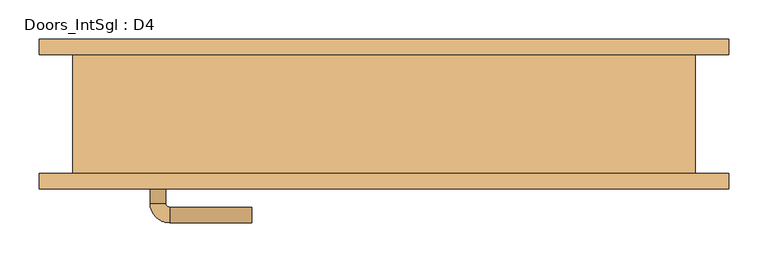
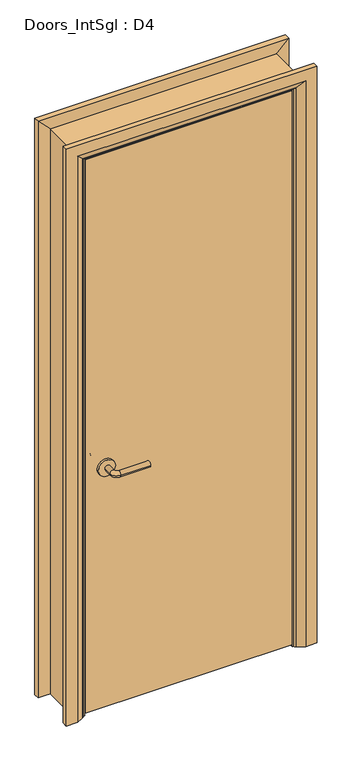
"""IFC4 building model written with IfcOpenShell, lengths in millimetres: door geometry, Doors_IntSgl : D4."""

from ifc_helpers import new_model, si_unit, point, frame, frame_2d, origin, place, context, project, spatial, polyline, circle_curve, ellipse_curve, trimmed, segment, composite_curve, outline, extrude, faceted_brep, source, transform, mapped, element, save
from ifc_brep_helpers import plane_surface, cylinder_surface, revolved_surface, advanced_brep


def doors_intsgl_d4_c85c0d06(model_context):
    return source(origin(), model_context, "Body", "SolidModel", [
        advanced_brep(
        [(-299.4508, -30.2, 900.0), (-279.4508, -30.2, 900.0), (-299.4508, -0.2, 900.0), (-279.4508, -0.2, 900.0), (-274.4508, 4.8, 900.0), (-274.4508, 24.8, 900.0), (-169.4508, 24.8, 900.0), (-169.4508, 4.8, 900.0)],
        [
            (0, 1, circle_curve(frame((-289.4508, -30.2, 900.0), z_axis=(0.0, -1.0, 0.0), x_axis=(1.0, 0.0, 0.0)), 10.0)),
            (1, 0, circle_curve(frame((-289.4508, -30.2, 900.0), z_axis=(0.0, -1.0, 0.0), x_axis=(1.0, 0.0, 0.0)), 10.0)),
            (0, 2),
            (2, 3, circle_curve(frame((-289.4508, -0.2, 900.0), z_axis=(0.0, -1.0, 0.0), x_axis=(1.0, 0.0, 0.0)), 10.0)),
            (3, 1),
            (3, 2, circle_curve(frame((-289.4508, -0.2, 900.0), z_axis=(0.0, -1.0, 0.0), x_axis=(1.0, 0.0, 0.0)), 10.0)),
            (4, 3, circle_curve(frame((-274.4508, -0.2, 900.0), z_axis=(0.0, 0.0, 1.0), x_axis=(-1.0, 0.0, 0.0)), 5.0)),
            (2, 5, circle_curve(frame((-274.4508, -0.2, 900.0), z_axis=(0.0, 0.0, -1.0), x_axis=(-1.0, 0.0, 0.0)), 25.0)),
            (5, 4, circle_curve(frame((-274.4508, 14.8, 900.0), z_axis=(-1.0, 0.0, 0.0), x_axis=(0.0, -1.0, 0.0)), 10.0)),
            (4, 5, circle_curve(frame((-274.4508, 14.8, 900.0), z_axis=(-1.0, 0.0, 0.0), x_axis=(0.0, -1.0, 0.0)), 10.0)),
            (6, 7, circle_curve(frame((-169.4508, 14.8, 900.0), z_axis=(1.0, 0.0, 0.0), x_axis=(0.0, -1.0, 0.0)), 10.0)),
            (7, 6, circle_curve(frame((-169.4508, 14.8, 900.0), z_axis=(1.0, 0.0, 0.0), x_axis=(0.0, -1.0, 0.0)), 10.0)),
            (5, 6),
            (7, 4),
        ],
        [
            plane_surface(frame((-289.4508, -30.2, 900.0), z_axis=(0.0, -1.0, 0.0), x_axis=(0.0, 0.0, 1.0))),
            cylinder_surface(frame((-289.4508, -30.2, 900.0), z_axis=(0.0, -1.0, 0.0), x_axis=(1.0, 0.0, 0.0)), 10.0),
            revolved_surface(trimmed(ellipse_curve(frame((-289.4508, -0.2, 900.0), z_axis=(0.0, -1.0, 0.0), x_axis=(1.0, 0.0, 0.0)), 10.0, 10.0), [point((-299.4508, -0.2, 900.0))], [point((-279.4508, -0.2, 900.0))], True, "CARTESIAN"), (-274.4508, -0.2, 900.0), (0.0, 0.0, -1.0)),
            revolved_surface(trimmed(ellipse_curve(frame((-289.4508, -0.2, 900.0), z_axis=(0.0, -1.0, 0.0), x_axis=(1.0, 0.0, 0.0)), 10.0, 10.0), [point((-279.4508, -0.2, 900.0))], [point((-299.4508, -0.2, 900.0))], True, "CARTESIAN"), (-274.4508, -0.2, 900.0), (0.0, 0.0, -1.0)),
            plane_surface(frame((-169.4508, 14.8, 900.0), z_axis=(1.0, 0.0, 0.0), x_axis=(0.0, 0.0, 1.0))),
            cylinder_surface(frame((-274.4508, 14.8, 900.0), z_axis=(-1.0, 0.0, 0.0), x_axis=(0.0, -1.0, 0.0)), 10.0),
        ],
        [
            (0, [[1, 2]]),
            (1, [[-1, 3, 4, 5]]),
            (1, [[-2, -5, 6, -3]]),
            (2, [[7, -4, 8, 9]]),
            (3, [[-8, -6, -7, 10]]),
            (4, [[11, 12]]),
            (5, [[-9, 13, -12, 14]]),
            (5, [[-10, -14, -11, -13]]),
        ],
    ),
        extrude(outline(composite_curve([segment(trimmed(circle_curve(frame_2d((900.0, -291.9508)), 30.0), [point((900.0, -321.9508))], [point((900.0, -261.9508))], False, "CARTESIAN"), True, "CONTINUOUS"), segment(trimmed(circle_curve(frame_2d((900.0, -291.9508)), 30.0), [point((900.0, -261.9508))], [point((900.0, -321.9508))], False, "CARTESIAN"), True, "CONTINUOUS")], self_intersect=False)), frame((0.0, -38.2, 0.0), z_axis=(0.0, 1.0, 0.0), x_axis=(0.0, 0.0, 1.0)), (0.0, 0.0, 1.0), 8.0),
        advanced_brep(
        [(-299.4508, -84.2, 900.0), (-279.4508, -84.2, 900.0), (-279.4508, -114.2, 900.0), (-299.4508, -114.2, 900.0), (-274.4508, -119.2, 900.0), (-274.4508, -139.2, 900.0), (-169.4508, -139.2, 900.0), (-169.4508, -119.2, 900.0)],
        [
            (0, 1, circle_curve(frame((-289.4508, -84.2, 900.0), z_axis=(0.0, 1.0, 0.0), x_axis=(1.0, 0.0, 0.0)), 10.0)),
            (1, 0, circle_curve(frame((-289.4508, -84.2, 900.0), z_axis=(0.0, 1.0, 0.0), x_axis=(1.0, 0.0, 0.0)), 10.0)),
            (1, 2),
            (2, 3, circle_curve(frame((-289.4508, -114.2, 900.0), z_axis=(0.0, 1.0, 0.0), x_axis=(1.0, 0.0, 0.0)), 10.0)),
            (3, 0),
            (3, 2, circle_curve(frame((-289.4508, -114.2, 900.0), z_axis=(0.0, 1.0, 0.0), x_axis=(1.0, 0.0, 0.0)), 10.0)),
            (4, 5, circle_curve(frame((-274.4508, -129.2, 900.0), z_axis=(-1.0, 0.0, 0.0), x_axis=(0.0, 1.0, 0.0)), 10.0)),
            (5, 3, circle_curve(frame((-274.4508, -114.2, 900.0), z_axis=(0.0, 0.0, -1.0), x_axis=(-1.0, 0.0, 0.0)), 25.0)),
            (2, 4, circle_curve(frame((-274.4508, -114.2, 900.0), z_axis=(0.0, 0.0, 1.0), x_axis=(-1.0, 0.0, 0.0)), 5.0)),
            (5, 4, circle_curve(frame((-274.4508, -129.2, 900.0), z_axis=(-1.0, 0.0, 0.0), x_axis=(0.0, 1.0, 0.0)), 10.0)),
            (6, 7, circle_curve(frame((-169.4508, -129.2, 900.0), z_axis=(1.0, 0.0, 0.0), x_axis=(0.0, 1.0, 0.0)), 10.0)),
            (7, 6, circle_curve(frame((-169.4508, -129.2, 900.0), z_axis=(1.0, 0.0, 0.0), x_axis=(0.0, 1.0, 0.0)), 10.0)),
            (4, 7),
            (6, 5),
        ],
        [
            plane_surface(frame((-289.4508, -84.2, 900.0), z_axis=(0.0, 1.0, 0.0), x_axis=(0.0, 0.0, 1.0))),
            cylinder_surface(frame((-289.4508, -84.2, 900.0), z_axis=(0.0, 1.0, 0.0), x_axis=(1.0, 0.0, 0.0)), 10.0),
            revolved_surface(trimmed(ellipse_curve(frame((-289.4508, -114.2, 900.0), z_axis=(0.0, -1.0, 0.0), x_axis=(1.0, 0.0, 0.0)), 10.0, 10.0), [point((-299.4508, -114.2, 900.0))], [point((-279.4508, -114.2, 900.0))], True, "CARTESIAN"), (-274.4508, -114.2, 900.0), (0.0, 0.0, -1.0)),
            revolved_surface(trimmed(ellipse_curve(frame((-289.4508, -114.2, 900.0), z_axis=(0.0, -1.0, 0.0), x_axis=(1.0, 0.0, 0.0)), 10.0, 10.0), [point((-279.4508, -114.2, 900.0))], [point((-299.4508, -114.2, 900.0))], True, "CARTESIAN"), (-274.4508, -114.2, 900.0), (0.0, 0.0, -1.0)),
            plane_surface(frame((-169.4508, -129.2, 900.0), z_axis=(1.0, 0.0, 0.0), x_axis=(0.0, 0.0, 1.0))),
            cylinder_surface(frame((-274.4508, -129.2, 900.0), z_axis=(-1.0, 0.0, 0.0), x_axis=(0.0, 1.0, 0.0)), 10.0),
        ],
        [
            (0, [[1, 2]]),
            (1, [[3, 4, 5, -2]]),
            (1, [[-5, 6, -3, -1]]),
            (2, [[7, 8, -4, 9]]),
            (3, [[10, -9, -6, -8]]),
            (4, [[11, 12]]),
            (5, [[13, -11, 14, -7]]),
            (5, [[-14, -12, -13, -10]]),
        ],
    ),
        extrude(outline(composite_curve([segment(trimmed(circle_curve(frame_2d((900.0, -291.9508)), 30.0), [point((900.0, -321.9508))], [point((900.0, -261.9508))], False, "CARTESIAN"), True, "CONTINUOUS"), segment(trimmed(circle_curve(frame_2d((900.0, -291.9508)), 30.0), [point((900.0, -261.9508))], [point((900.0, -321.9508))], False, "CARTESIAN"), True, "CONTINUOUS")], self_intersect=False)), frame((0.0, -84.2, 0.0), z_axis=(0.0, 1.0, 0.0), x_axis=(0.0, 0.0, 1.0)), (0.0, 0.0, 1.0), 8.0),
        extrude(outline(polyline([(364.4508, -38.2), (364.4508, -76.2), (-364.4508, -76.2), (-364.4508, -38.2), (364.4508, -38.2)])), frame((0.0, 0.0, 8.0), z_axis=(0.0, 0.0, 1.0), x_axis=(1.0, 0.0, 0.0)), (0.0, 0.0, 1.0), 2060.0),
        advanced_brep(
        [(441.4508, -96.2, 0.0), (401.4508, -96.2, 0.0), (375.4508, -82.2, 0.0), (371.4508, -76.2, 0.0), (441.4508, -76.2, 0.0), (441.4508, -76.2, 2145.0), (441.4508, -96.2, 2145.0), (371.4508, -76.2, 2075.0), (-371.4508, -76.2, 2075.0), (-371.4508, -76.2, 0.0), (-441.4508, -76.2, 0.0), (-441.4508, -76.2, 2145.0), (375.4508, -82.2, 2079.0), (401.4508, -96.2, 2105.0), (-441.4508, -96.2, 2145.0), (-441.4508, -96.2, 0.0), (-401.4508, -96.2, 0.0), (-401.4508, -96.2, 2105.0), (-375.4508, -82.2, 0.0), (-375.4508, -82.2, 2079.0)],
        [
            (0, 1),
            (1, 2),
            (2, 3, circle_curve(frame((379.4508, -75.2, 0.0), z_axis=(0.0, 0.0, -1.0), x_axis=(1.0, 0.0, 0.0)), 8.0622577)),
            (3, 4),
            (4, 0),
            (4, 5),
            (5, 6),
            (6, 0),
            (3, 7),
            (7, 8),
            (8, 9),
            (9, 10),
            (10, 11),
            (11, 5),
            (2, 12),
            (12, 7, ellipse_curve(frame((379.4508, -75.2, 2083.0), z_axis=(0.7071067811865475, 0.0, -0.7071067811865475), x_axis=(-0.7071067811865474, 0.0, -0.7071067811865476)), 11.4017543, 8.0622577)),
            (1, 13),
            (13, 12),
            (6, 14),
            (14, 15),
            (15, 16),
            (16, 17),
            (17, 13),
            (10, 15),
            (14, 11),
            (9, 18, circle_curve(frame((-379.4508, -75.2, 0.0), z_axis=(0.0, 0.0, -1.0), x_axis=(-1.0, 0.0, 0.0)), 8.0622577)),
            (18, 16),
            (19, 18),
            (8, 19, ellipse_curve(frame((-379.4508, -75.2, 2083.0), z_axis=(-0.7071067811865475, 0.0, -0.7071067811865475), x_axis=(-0.7071067811865474, 0.0, 0.7071067811865476)), 11.4017543, 8.0622577)),
            (19, 17),
            (12, 19),
        ],
        [
            plane_surface(frame((371.4508, -76.2, 0.0), z_axis=(0.0, 0.0, -1.0), x_axis=(0.0, 1.0, 0.0))),
            plane_surface(frame((441.4508, -96.2, 0.0), z_axis=(1.0, 0.0, 0.0), x_axis=(0.0, 0.0, 1.0))),
            plane_surface(frame((441.4508, -76.2, 0.0), z_axis=(0.0, 1.0, 0.0), x_axis=(0.0, 0.0, 1.0))),
            cylinder_surface(frame((379.4508, -75.2, 0.0), z_axis=(0.0, 0.0, -1.0), x_axis=(1.0, 0.0, 0.0)), 8.0622577),
            plane_surface(frame((375.4508, -82.2, 0.0), z_axis=(-0.4740998230350126, -0.880471099922178, 0.0), x_axis=(0.0, 0.0, 1.0))),
            plane_surface(frame((401.4508, -96.2, 0.0), z_axis=(0.0, -1.0, 0.0), x_axis=(0.0, 0.0, 1.0))),
            plane_surface(frame((-441.4508, -96.2, 2145.0), z_axis=(-1.0, 0.0, 0.0), x_axis=(0.0, 0.0, -1.0))),
            plane_surface(frame((-371.4508, -76.2, 0.0), z_axis=(0.0, 0.0, -1.0), x_axis=(0.0, 1.0, 0.0))),
            cylinder_surface(frame((-379.4508, -75.2, 2075.0), z_axis=(0.0, 0.0, 1.0), x_axis=(-1.0, 0.0, 0.0)), 8.0622577),
            plane_surface(frame((-375.4508, -82.2, 2079.0), z_axis=(0.47409982303501824, -0.8804710999221749, 0.0), x_axis=(0.0, 0.0, -1.0))),
            plane_surface(frame((441.4508, -96.2, 2145.0), z_axis=(0.0, 0.0, 1.0), x_axis=(-1.0, 0.0, 0.0))),
            cylinder_surface(frame((371.4508, -75.2, 2083.0), z_axis=(1.0, 0.0, 0.0), x_axis=(0.0, 0.0, 1.0)), 8.0622577),
            plane_surface(frame((375.4508, -82.2, 2079.0), z_axis=(0.0, -0.8804710999221764, -0.4740998230350154), x_axis=(-1.0, 0.0, 0.0))),
        ],
        [
            (0, [[1, 2, 3, 4, 5]]),
            (1, [[6, 7, 8, -5]]),
            (2, [[9, 10, 11, 12, 13, 14, -6, -4]]),
            (3, [[15, 16, -9, -3]]),
            (4, [[17, 18, -15, -2]]),
            (5, [[-8, 19, 20, 21, 22, 23, -17, -1]]),
            (6, [[-13, 24, -20, 25]]),
            (7, [[-24, -12, 26, 27, -21]]),
            (8, [[28, -26, -11, 29]]),
            (9, [[-22, -27, -28, 30]]),
            (10, [[-14, -25, -19, -7]]),
            (11, [[31, -29, -10, -16]]),
            (12, [[-23, -30, -31, -18]]),
        ],
    ),
        extrude(outline(polyline([(0.0, -347.4508), (2051.0, -347.4508), (2051.0, 347.4508), (0.0, 347.4508), (0.0, 366.4508), (2070.0, 366.4508), (2070.0, -366.4508), (0.0, -366.4508), (0.0, -347.4508)])), frame((0.0, -36.2, 0.0), z_axis=(0.0, 1.0, 0.0), x_axis=(0.0, 0.0, 1.0)), (0.0, 0.0, 1.0), 32.0),
        advanced_brep(
        [(-441.4508, 96.2, 0.0), (-401.4508, 96.2, 0.0), (-375.4508, 82.2, 0.0), (-371.4508, 76.2, 0.0), (-441.4508, 76.2, 0.0), (-441.4508, 76.2, 2145.0), (-441.4508, 96.2, 2145.0), (-371.4508, 76.2, 2075.0), (-375.4508, 82.2, 2079.0), (-401.4508, 96.2, 2105.0), (441.4508, 96.2, 0.0), (441.4508, 76.2, 0.0), (371.4508, 76.2, 0.0), (375.4508, 82.2, 0.0), (401.4508, 96.2, 0.0), (441.4508, 96.2, 2145.0), (401.4508, 96.2, 2105.0), (375.4508, 82.2, 2079.0), (371.4508, 76.2, 2075.0), (441.4508, 76.2, 2145.0)],
        [
            (0, 1),
            (1, 2),
            (2, 3, circle_curve(frame((-379.4508, 75.2, 0.0), z_axis=(0.0, 0.0, -1.0), x_axis=(-1.0, 0.0, 0.0)), 8.0622577)),
            (3, 4),
            (4, 0),
            (4, 5),
            (5, 6),
            (6, 0),
            (3, 7),
            (7, 5),
            (2, 8),
            (8, 7, ellipse_curve(frame((-379.4508, 75.2, 2083.0), z_axis=(-0.7071067811865475, 0.0, -0.7071067811865475), x_axis=(0.7071067811865474, 0.0, -0.7071067811865476)), 11.4017543, 8.0622577)),
            (1, 9),
            (9, 8),
            (6, 9),
            (10, 11),
            (11, 12),
            (12, 13, circle_curve(frame((379.4508, 75.2, 0.0), z_axis=(0.0, 0.0, -1.0), x_axis=(1.0, 0.0, 0.0)), 8.0622577)),
            (13, 14),
            (14, 10),
            (15, 10),
            (14, 16),
            (16, 15),
            (13, 17),
            (17, 16),
            (12, 18),
            (18, 17, ellipse_curve(frame((379.4508, 75.2, 2083.0), z_axis=(0.7071067811865475, 0.0, -0.7071067811865475), x_axis=(0.7071067811865474, 0.0, 0.7071067811865476)), 11.4017543, 8.0622577)),
            (11, 19),
            (19, 18),
            (15, 19),
            (5, 19),
            (15, 6),
            (7, 18),
            (8, 17),
            (9, 16),
        ],
        [
            plane_surface(frame((-371.4508, 149.0010989, 0.0), z_axis=(0.0, 0.0, -1.0), x_axis=(1.0, 0.0, 0.0))),
            plane_surface(frame((-441.4508, 96.2, 0.0), z_axis=(-1.0, 0.0, 0.0), x_axis=(0.0, 0.0, 1.0))),
            plane_surface(frame((-441.4508, 76.2, 0.0), z_axis=(0.0, -1.0, 0.0), x_axis=(0.0, 0.0, 1.0))),
            cylinder_surface(frame((-379.4508, 75.2, 0.0), z_axis=(0.0, 0.0, -1.0), x_axis=(-1.0, 0.0, 0.0)), 8.0622577),
            plane_surface(frame((-375.4508, 82.2, 0.0), z_axis=(0.4740998230350183, 0.8804710999221749, 0.0), x_axis=(0.0, 0.0, 1.0))),
            plane_surface(frame((-401.4508, 96.2, 0.0), z_axis=(0.0, 1.0, 0.0), x_axis=(0.0, 0.0, 1.0))),
            plane_surface(frame((371.4508, 149.0010989, 0.0), z_axis=(0.0, 0.0, -1.0), x_axis=(-1.0, 0.0, 0.0))),
            plane_surface(frame((401.4508, 96.2, 2105.0), z_axis=(0.0, 1.0, 0.0), x_axis=(0.0, 0.0, -1.0))),
            plane_surface(frame((375.4508, 82.2, 2079.0), z_axis=(-0.4740998230350183, 0.8804710999221749, 0.0), x_axis=(0.0, 0.0, -1.0))),
            cylinder_surface(frame((379.4508, 75.2, 2075.0), z_axis=(0.0, 0.0, 1.0), x_axis=(1.0, 0.0, 0.0)), 8.0622577),
            plane_surface(frame((441.4508, 76.2, 2145.0), z_axis=(0.0, -1.0, 0.0), x_axis=(0.0, 0.0, -1.0))),
            plane_surface(frame((441.4508, 96.2, 2145.0), z_axis=(1.0, 0.0, 0.0), x_axis=(0.0, 0.0, -1.0))),
            plane_surface(frame((-441.4508, 96.2, 2145.0), z_axis=(0.0, 0.0, 1.0), x_axis=(1.0, 0.0, 0.0))),
            plane_surface(frame((-441.4508, 76.2, 2145.0), z_axis=(0.0, -1.0, 0.0), x_axis=(1.0, 0.0, 0.0))),
            cylinder_surface(frame((-371.4508, 75.2, 2083.0), z_axis=(-1.0, 0.0, 0.0), x_axis=(0.0, 0.0, 1.0)), 8.0622577),
            plane_surface(frame((-375.4508, 82.2, 2079.0), z_axis=(0.0, 0.8804710999221749, -0.4740998230350183), x_axis=(1.0, 0.0, 0.0))),
            plane_surface(frame((-401.4508, 96.2, 2105.0), z_axis=(0.0, 1.0, 0.0), x_axis=(1.0, 0.0, 0.0))),
        ],
        [
            (0, [[1, 2, 3, 4, 5]]),
            (1, [[6, 7, 8, -5]]),
            (2, [[9, 10, -6, -4]]),
            (3, [[11, 12, -9, -3]]),
            (4, [[13, 14, -11, -2]]),
            (5, [[-8, 15, -13, -1]]),
            (6, [[16, 17, 18, 19, 20]]),
            (7, [[21, -20, 22, 23]]),
            (8, [[-22, -19, 24, 25]]),
            (9, [[-24, -18, 26, 27]]),
            (10, [[-26, -17, 28, 29]]),
            (11, [[-28, -16, -21, 30]]),
            (12, [[31, -30, 32, -7]]),
            (13, [[33, -29, -31, -10]]),
            (14, [[34, -27, -33, -12]]),
            (15, [[35, -25, -34, -14]]),
            (16, [[-32, -23, -35, -15]]),
        ],
    ),
        faceted_brep([(-366.4508, -76.2, 0.0), (-398.4508, -76.2, 0.0), (-398.4508, 76.2, 0.0), (-366.4508, 76.2, 0.0), (-366.4508, 76.2, 2070.0), (-366.4508, -76.2, 2070.0), (-398.4508, 76.2, 2102.0), (-398.4508, -76.2, 2102.0), (366.4508, -76.2, 0.0), (366.4508, 76.2, 0.0), (398.4508, 76.2, 0.0), (398.4508, -76.2, 0.0), (366.4508, -76.2, 2070.0), (398.4508, -76.2, 2102.0), (398.4508, 76.2, 2102.0), (366.4508, 76.2, 2070.0)], [[[0, 1, 2, 3]], [[3, 4, 5, 0]], [[2, 6, 4, 3]], [[1, 7, 6, 2]], [[0, 5, 7, 1]], [[8, 9, 10, 11]], [[12, 8, 11, 13]], [[13, 11, 10, 14]], [[14, 10, 9, 15]], [[15, 9, 8, 12]], [[4, 15, 12, 5]], [[6, 14, 15, 4]], [[7, 13, 14, 6]], [[5, 12, 13, 7]]]),
    ])


if __name__ == "__main__":
    model = new_model("IFC4")
    model_context = context("Model", 3, world=origin())
    ifc_project = project(units=[si_unit("LENGTHUNIT", "METRE", prefix="MILLI")], contexts=[model_context])
    site = spatial("IfcSite", under=ifc_project)
    building = spatial("IfcBuilding", under=site)
    placement = place(None, origin())
    doors_intsgl_d4_shape = doors_intsgl_d4_c85c0d06(model_context)
    element("IfcDoor", 1, ObjectType="Doors_IntSgl : D4", at=placement, inside=building, context=model_context, shape_type="MappedRepresentation", body=[
        mapped(doors_intsgl_d4_shape, transform((0.0, 0.0, 0.0), x_axis=(1.0, 0.0, 0.0), y_axis=(0.0, 1.0, 0.0), z_axis=(0.0, 0.0, 1.0))),
    ])
    save(model, "model.ifc")

# Revit data of these elements
# Type "Doors_IntSgl : D4"
#   Type Mark = "50"
#   Type Comments = "Internal Single"
#   Operation = "SingleSwingRight"
#   Manufacturer = "Revit"
#   Keynote = "L20"
#   Description = "Internal Single Door"
#   Analytic Construction = "Metal"
#   UnderCut = 0.026247 ft
#   Tolerance = 0.006562 ft
#   Thickness = 0.124672 ft
#   Thermal Resistance (R) = 0.270117 (m²·K)/W
#   Structural Tolerance = 0.026247 ft
#   StopDepth = 0.104987 ft
#   Stop Thickness = 0.062336 ft
#   Rough Width = 2.667 ft
#   Rough Height = 6.922572 ft
#   Height to Top Lock Rail = 3.28084 ft
#   Heat Transfer Coefficient (U) = 3.7021 W/(m²·K)
#   Handle Z Distance = 2.952756 ft
#   Handle X Distance = 0.246063 ft
#   Frame Thickness = 0.104987 ft
#   Door Panel Width = 2.391409 ft
#   Door Panel Thickness = 0.124672 ft
#   Door Panel Offset = 0.0 ft
#   Height = 6.922572 ft
#   Width = 2.667 ft
#   Door Panel Height = 6.75853 ft
#   Architrave Setback = 0.016404 ft
#   Vis - Ironmongery = yes
#   Material Ironmongery = Door - Handle
#   Material Frame = Door - Frame/Mullion (1)
#   Material Door = Door - Panel
#   Material Architrave = Door - Architrave
#   Visual Light Transmittance = 0
#   Solar Heat Gain Coefficient = 0
#   Function = (empty or 0)
#   Wall Closure = (empty or 0)
# Element 1 (IfcDoor, "Doors_IntSgl : D4")
#   Materials on its faces: "Door - Architrave", "Door - Handle", "Door - Frame/Mullion (1)", "Door - Panel"
# Materials
#   "Door - Handle": colour RGB 0 0 0, transparency 0, Keynote = "P21", Cost = 0
#   "Door - Frame/Mullion (1)": class "Wood", colour RGB 212 179 113, transparency 0, Keynote = "L20", Cost = 0
#   "Door - Panel": class "Wood", colour RGB 210 159 95, transparency 0, Keynote = "L20", Cost = 0
#   "Door - Architrave": class "Wood", colour RGB 154 90 5, transparency 0, Keynote = "P20", Cost = 0
